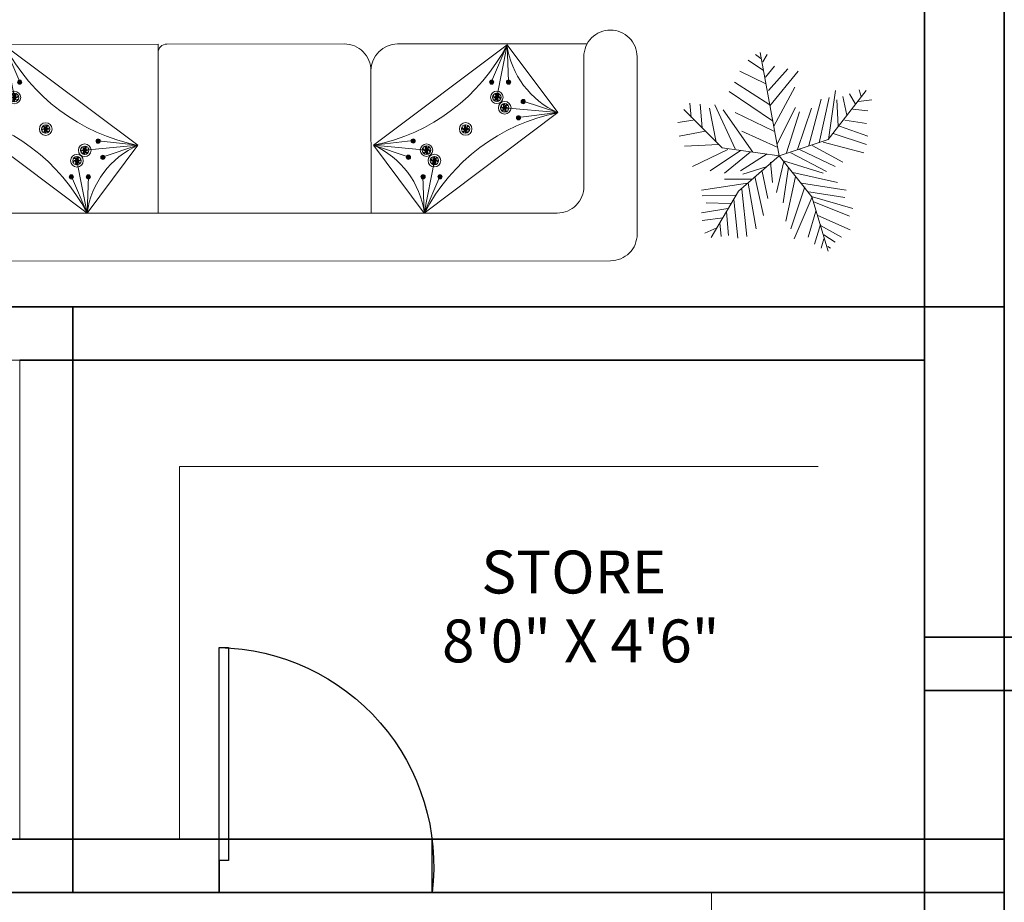
# Model space of a CAD drawing. Units: inches. Extents: x -61 to 1599, y -1316 to 257.
# Tile 23 of 204: x 434 to 545, y -1011 to -912. Entities that reach past the tile are written whole.
import ezdxf

# ---------------------------------------------------------------- set-up
doc = ezdxf.new("R2010")
doc.units = ezdxf.units.IN
doc.header["$MEASUREMENT"] = 0
doc.linetypes.add('ACAD_ISO02W100', pattern=[15, 12, -3])
for name, color, linetype, lineweight in [('A-ANNO-DIMS', 2, 'Continuous', 18), ('A-AREA-IDEN', 1, 'Continuous', 18), ('A-FLOR-CASE', 8, 'Continuous', 18), ('A-WALL-JAMB', 4, 'ACAD_ISO02W100', 25), ('DOORS', 2, 'Continuous', 25), ('FURNITURE', 83, 'Continuous', 18), ('WALLS', 4, 'Continuous', 35)]:
    doc.layers.add(name, color=color, linetype=linetype, lineweight=lineweight)
doc.layers.add('FUR', color=83, linetype='Continuous')
doc.styles.get("Standard").update_dxf_attribs({"font": 'arial.ttf'})
doc.dimstyles.get("Standard").update_dxf_attribs({"dimtxt": 0.18, "dimasz": 0.18, "dimexe": 0.18, "dimexo": 0.0625, "dimgap": 0.09, "dimtad": 0, "dimtih": 1, "dimtoh": 1, "dimdec": 0, "dimzin": 0, "dimdsep": 46, "dimlunit": 3, "dimtxsty": 'Standard', "dimcen": 0.09, "dimadec": 0, "dimazin": 0, "dimtfac": 1, "dimtdec": 0, "dimtofl": 0, "dimtmove": 0, "dimatfit": 3, "dimfxl": 1, "dimtolj": 1, "dimtzin": 0, "dimarcsym": 0})

# ---------------------------------------------------------------- blocks, each defined once
blk = doc.blocks.new('*U264')
for p, q in [((-10.186, 53.64), (-13.084, 55.962)), ((0, 0), (-10.5, 57)), ((-9.099, 51.782), (-6.563, 55.962)), ((-8.737, 47.138), (-17.069, 52.711)), ((-7.65, 43.423), (-2.578, 49.46)), ((-7.288, 39.707), (-21.778, 46.673)), ((-5.839, 35.992), (4.667, 48.067)), ((-5.114, 27.632), (10.463, 46.673)), ((-5.114, 28.097), (-24.676, 40.636)), ((-3.665, 19.273), (-27.574, 35.527)), ((-2.941, 16.486), (8.652, 37.85)), ((27, 9), (48, 36)), ((27.127, 9.056), (31.112, 35.992)), ((35.096, 32.741), (37.27, 22.524)), ((38.719, 34.134), (41.979, 28.561)), ((44.153, 36.456), (45.239, 32.741)), ((-48.585, 21.131), (-49.309, 29.026)), ((-43.513, 28.561), (-42.427, 15.558)), ((-35.544, 28.097), (-24.314, 3.947)), ((16.259, 5.805), (23.142, 31.348)), ((22.055, 7.198), (27.489, 32.277)), ((31.836, 30.883), (32.561, 16.486)), ((43.791, 29.954), (51.036, 30.883)), ((-31.5, 4.5), (-52.5, 25.5)), ((-38.442, 26.239), (-34.819, 7.663)), ((-14.533, 2.09), (-30.834, 25.31)), ((-24.314, 23.917), (-2.941, 13.7)), ((-1.129, 6.734), (9.014, 26.704)), ((3.942, 1.625), (11.187, 24.381)), ((10.101, 3.483), (17.708, 26.239)), ((40.53, 25.775), (48.862, 24.846)), ((-47.498, 19.737), (-55.83, 18.344)), ((33.285, 16.486), (48.862, 10.913)), ((36.183, 19.737), (48.137, 17.88)), ((-40.615, 13.7), (-55.105, 10.913)), ((-20.691, 13.7), (-1.129, 4.876)), ((29.662, 12.307), (48.137, 6.269)), ((-33.37, 6.269), (-52.207, 5.34)), ((0, 0), (27, 9)), ((18.07, 5.805), (35.096, -3.483)), ((24.229, 7.663), (46.688, 1.625)), ((-28.299, 3.483), (-47.86, -5.805)), ((-21.416, 3.018), (-38.079, -8.128)), ((0, 0), (-31.5, 4.5)), ((-15.982, 2.09), (-30.11, -9.521)), ((0, 0), (-22.5, -19.5)), ((-6.563, 1.161), (-21.416, -8.128)), ((0, 0), (18, -22.5)), ((6.478, 1.625), (26.04, -8.592)), ((11.187, 3.483), (30.749, -5.805)), ((-4.752, -3.483), (-3.665, -14.629)), ((2.493, -3.019), (-1.491, -20.202)), ((1.769, -2.555), (24.229, -9.521)), ((-6.563, -5.805), (-19.967, -9.985)), ((-9.461, -8.592), (-6.201, -23.453)), ((5.029, -6.27), (2.131, -25.775)), ((7.565, -9.056), (32.198, -14.629)), ((-17.431, -15.094), (-42.789, -18.809)), ((-15.257, -12.772), (-30.11, -12.772)), ((-17.069, -15.094), (-12.721, -40.172)), ((-13.446, -11.378), (-8.737, -32.741)), ((9.014, -11.378), (3.58, -35.992)), ((12.274, -15.094), (36.907, -18.809)), ((-24.314, -21.596), (-42.427, -22.06)), ((-22.5, -19.5), (-37.5, -45)), ((-20.691, -18.345), (-17.793, -44.352)), ((14.085, -16.951), (6.478, -40.172)), ((16.259, -19.738), (36.183, -22.989)), ((-26.849, -26.24), (-40.253, -25.775)), ((-25.038, -23.918), (-22.865, -45.281)), ((18.07, -22.524), (8.289, -45.745)), ((18, -22.5), (27, -52.5)), ((18.433, -22.524), (40.53, -29.026)), ((19.157, -25.311), (38.719, -33.206)), ((-28.299, -29.026), (-42.789, -31.348)), ((-29.023, -30.884), (-27.936, -43.887)), ((20.244, -30.419), (15.897, -44.816)), ((-30.834, -34.135), (-42.427, -35.528)), ((-32.646, -36.921), (-31.921, -44.352)), ((22.78, -37.85), (19.519, -48.532)), ((21.331, -32.741), (39.081, -40.636)), ((-34.457, -39.708), (-40.978, -42.494)), ((22.78, -38.314), (34.372, -44.816)), ((24.591, -45.745), (23.142, -50.854)), ((24.591, -43.423), (30.749, -47.603)), ((26.764, -49.925), (28.213, -50.854))]:
    blk.add_line(p, q)
blk = doc.blocks.new('DOOR-SWING-24')
blk.add_line((0, 0), (0, 3.6))
blk.add_lwpolyline([(0, 0), (0, -24), (1.05, -24), (1.05, 0)], close=True)
blk.add_arc((-0.44, 0.62), 24.62, 271.0259, 6.9559)
blk = doc.blocks.new('*U514')
at = {"layer": 'FUR'}
blk.add_open_spline([(0, 0.08), (-0.03, 0.05), (-0.1, -0.02), (0.08, -0.02), (0.02, -0.06), (0, -0.08)], degree=3, knots=[0, 0, 0, 0, 0.0954578, 0.1898773, 0.2470677, 0.2470677, 0.2470677, 0.2470677], dxfattribs=at)
blk = doc.blocks.new('*U515')
at = {"layer": 'FUR', "transparency": 16777216}
for p, rotation in [((222.17, -79.98), 60), ((222.31, -79.97), 300), ((222.18, -80.06), 120), ((222.25, -80.09), 180), ((222.32, -80.05), 240)]:
    blk.add_blockref('*U514', p, dxfattribs=dict(at, rotation=rotation))
blk.add_blockref('*U514', (222.24, -79.93), dxfattribs=at)
blk = doc.blocks.new('*U516')
at = {"layer": 'FUR'}
blk.add_open_spline([(0, 0.08), (-0.03, 0.05), (-0.1, -0.02), (0.08, -0.02), (0.02, -0.06), (0, -0.08)], degree=3, knots=[0, 0, 0, 0, 0.0954578, 0.1898773, 0.2470677, 0.2470677, 0.2470677, 0.2470677], dxfattribs=at)
blk = doc.blocks.new('*U517')
at = {"layer": 'FUR', "transparency": 16777216}
for p, rotation in [((222.17, -79.98), 60), ((222.31, -79.97), 300), ((222.18, -80.06), 120), ((222.25, -80.09), 180), ((222.32, -80.05), 240)]:
    blk.add_blockref('*U516', p, dxfattribs=dict(at, rotation=rotation))
blk.add_blockref('*U516', (222.24, -79.93), dxfattribs=at)
blk = doc.blocks.new('*U510')
at = {"layer": 'FUR'}
blk.add_open_spline([(0, 0.08), (-0.03, 0.05), (-0.1, -0.02), (0.08, -0.02), (0.02, -0.06), (0, -0.08)], degree=3, knots=[0, 0, 0, 0, 0.0954578, 0.1898773, 0.2470677, 0.2470677, 0.2470677, 0.2470677], dxfattribs=at)
blk = doc.blocks.new('*U511')
at = {"layer": 'FUR', "transparency": 16777216}
for p, rotation in [((222.17, -79.98), 60), ((222.31, -79.97), 300), ((222.18, -80.06), 120), ((222.25, -80.09), 180), ((222.32, -80.05), 240)]:
    blk.add_blockref('*U510', p, dxfattribs=dict(at, rotation=rotation))
blk.add_blockref('*U510', (222.24, -79.93), dxfattribs=at)
blk = doc.blocks.new('*U479')
at = {"layer": 'FUR'}
blk.add_open_spline([(0.01, 0.24), (-0.09, 0.14), (-0.29, -0.05), (0.22, -0.05), (0.07, -0.19), (0.01, -0.24)], degree=3, knots=[0, 0, 0, 0, 0.2846533, 0.5662105, 0.736751, 0.736751, 0.736751, 0.736751], dxfattribs=at)
blk = doc.blocks.new('*U480')
at = {"layer": 'FUR', "transparency": 16777216}
for p, rotation in [((662.52, -238.49), 60), ((662.53, -238.73), 120), ((662.74, -238.83), 180), ((662.93, -238.46), 300), ((662.94, -238.7), 240)]:
    blk.add_blockref('*U479', p, dxfattribs=dict(at, rotation=rotation))
blk.add_blockref('*U479', (662.72, -238.36), dxfattribs=at)
blk = doc.blocks.new('*U512')
at = {"layer": 'FUR'}
blk.add_open_spline([(0, 0.08), (-0.03, 0.05), (-0.1, -0.02), (0.08, -0.02), (0.02, -0.06), (0, -0.08)], degree=3, knots=[0, 0, 0, 0, 0.0954578, 0.1898773, 0.2470677, 0.2470677, 0.2470677, 0.2470677], dxfattribs=at)
blk = doc.blocks.new('*U513')
at = {"layer": 'FUR', "transparency": 16777216}
for p, rotation in [((222.17, -79.98), 60), ((222.31, -79.97), 300), ((222.18, -80.06), 120), ((222.25, -80.09), 180), ((222.32, -80.05), 240)]:
    blk.add_blockref('*U512', p, dxfattribs=dict(at, rotation=rotation))
blk.add_blockref('*U512', (222.24, -79.93), dxfattribs=at)
blk = doc.blocks.new('*U483')
at = {"layer": 'FUR'}
blk.add_open_spline([(0.01, 0.24), (-0.09, 0.14), (-0.29, -0.05), (0.22, -0.05), (0.07, -0.19), (0.01, -0.24)], degree=3, knots=[0, 0, 0, 0, 0.2846533, 0.5662105, 0.736751, 0.736751, 0.736751, 0.736751], dxfattribs=at)
blk = doc.blocks.new('*U484')
at = {"layer": 'FUR', "transparency": 16777216}
for p, rotation in [((662.52, -238.49), 60), ((662.53, -238.73), 120), ((662.74, -238.83), 180), ((662.93, -238.46), 300), ((662.94, -238.7), 240)]:
    blk.add_blockref('*U483', p, dxfattribs=dict(at, rotation=rotation))
blk.add_blockref('*U483', (662.72, -238.36), dxfattribs=at)
blk = doc.blocks.new('*U498')
at = {"layer": 'FUR'}
blk.add_open_spline([(0, 0.08), (-0.03, 0.05), (-0.1, -0.02), (0.08, -0.02), (0.02, -0.06), (0, -0.08)], degree=3, knots=[0, 0, 0, 0, 0.0954578, 0.1898773, 0.2470677, 0.2470677, 0.2470677, 0.2470677], dxfattribs=at)
blk = doc.blocks.new('*U499')
at = {"layer": 'FUR', "transparency": 16777216}
for p, rotation in [((222.17, -79.98), 60), ((222.31, -79.97), 300), ((222.18, -80.06), 120), ((222.25, -80.09), 180), ((222.32, -80.05), 240)]:
    blk.add_blockref('*U498', p, dxfattribs=dict(at, rotation=rotation))
blk.add_blockref('*U498', (222.24, -79.93), dxfattribs=at)
blk = doc.blocks.new('*U485')
at = {"layer": 'FUR'}
blk.add_open_spline([(0.01, 0.24), (-0.09, 0.14), (-0.29, -0.05), (0.22, -0.05), (0.07, -0.19), (0.01, -0.24)], degree=3, knots=[0, 0, 0, 0, 0.2846533, 0.5662105, 0.736751, 0.736751, 0.736751, 0.736751], dxfattribs=at)
blk = doc.blocks.new('*U497')
at = {"layer": 'FUR', "transparency": 16777216}
for p, rotation in [((662.52, -238.49), 60), ((662.53, -238.73), 120), ((662.74, -238.83), 180), ((662.93, -238.46), 300), ((662.94, -238.7), 240)]:
    blk.add_blockref('*U485', p, dxfattribs=dict(at, rotation=rotation))
blk.add_blockref('*U485', (662.72, -238.36), dxfattribs=at)
blk = doc.blocks.new('*U481')
at = {"layer": 'FUR'}
blk.add_open_spline([(0.01, 0.24), (-0.09, 0.14), (-0.29, -0.05), (0.22, -0.05), (0.07, -0.19), (0.01, -0.24)], degree=3, knots=[0, 0, 0, 0, 0.2846533, 0.5662105, 0.736751, 0.736751, 0.736751, 0.736751], dxfattribs=at)
blk = doc.blocks.new('*U482')
at = {"layer": 'FUR', "transparency": 16777216}
for p, rotation in [((662.52, -238.49), 60), ((662.53, -238.73), 120), ((662.74, -238.83), 180), ((662.93, -238.46), 300), ((662.94, -238.7), 240)]:
    blk.add_blockref('*U481', p, dxfattribs=dict(at, rotation=rotation))
blk.add_blockref('*U481', (662.72, -238.36), dxfattribs=at)
blk = doc.blocks.new('*U477')
at = {"layer": 'FUR'}
blk.add_open_spline([(0, 0.08), (-0.03, 0.05), (-0.1, -0.02), (0.08, -0.02), (0.02, -0.06), (0, -0.08)], degree=3, knots=[0, 0, 0, 0, 0.0954578, 0.1898773, 0.2470677, 0.2470677, 0.2470677, 0.2470677], dxfattribs=at)
blk = doc.blocks.new('*U478')
at = {"layer": 'FUR', "transparency": 16777216}
for p, rotation in [((222.17, -79.98), 60), ((222.31, -79.97), 300), ((222.18, -80.06), 120), ((222.25, -80.09), 180), ((222.32, -80.05), 240)]:
    blk.add_blockref('*U477', p, dxfattribs=dict(at, rotation=rotation))
blk.add_blockref('*U477', (222.24, -79.93), dxfattribs=at)
blk = doc.blocks.new('*U508')
at = {"layer": 'FUR'}
blk.add_open_spline([(0, 0.08), (-0.03, 0.05), (-0.1, -0.02), (0.08, -0.02), (0.02, -0.06), (0, -0.08)], degree=3, knots=[0, 0, 0, 0, 0.0954578, 0.1898773, 0.2470677, 0.2470677, 0.2470677, 0.2470677], dxfattribs=at)
blk = doc.blocks.new('*U509')
at = {"layer": 'FUR', "transparency": 16777216}
for p, rotation in [((222.17, -79.98), 60), ((222.31, -79.97), 300), ((222.18, -80.06), 120), ((222.25, -80.09), 180), ((222.32, -80.05), 240)]:
    blk.add_blockref('*U508', p, dxfattribs=dict(at, rotation=rotation))
blk.add_blockref('*U508', (222.24, -79.93), dxfattribs=at)
blk = doc.blocks.new('*U506')
at = {"layer": 'FUR'}
blk.add_open_spline([(0, 0.08), (-0.03, 0.05), (-0.1, -0.02), (0.08, -0.02), (0.02, -0.06), (0, -0.08)], degree=3, knots=[0, 0, 0, 0, 0.0954578, 0.1898773, 0.2470677, 0.2470677, 0.2470677, 0.2470677], dxfattribs=at)
blk = doc.blocks.new('*U507')
at = {"layer": 'FUR', "transparency": 16777216}
for p, rotation in [((222.17, -79.98), 60), ((222.31, -79.97), 300), ((222.18, -80.06), 120), ((222.25, -80.09), 180), ((222.32, -80.05), 240)]:
    blk.add_blockref('*U506', p, dxfattribs=dict(at, rotation=rotation))
blk.add_blockref('*U506', (222.24, -79.93), dxfattribs=at)
blk = doc.blocks.new('*U476')
at = {"layer": 'FUR'}
blk.add_open_spline([(0, 0.08), (-0.03, 0.05), (-0.1, -0.02), (0.08, -0.02), (0.02, -0.06), (0, -0.08)], degree=3, knots=[0, 0, 0, 0, 0.0954578, 0.1898773, 0.2470677, 0.2470677, 0.2470677, 0.2470677], dxfattribs=at)
blk = doc.blocks.new('*U489')
at = {"layer": 'FUR', "transparency": 16777216}
for p, rotation in [((222.17, -79.98), 60), ((222.31, -79.97), 300), ((222.18, -80.06), 120), ((222.25, -80.09), 180), ((222.32, -80.05), 240)]:
    blk.add_blockref('*U476', p, dxfattribs=dict(at, rotation=rotation))
blk.add_blockref('*U476', (222.24, -79.93), dxfattribs=at)
blk = doc.blocks.new('*U490')
at = {"layer": 'FUR'}
blk.add_open_spline([(0, 0.08), (-0.03, 0.05), (-0.1, -0.02), (0.08, -0.02), (0.02, -0.06), (0, -0.08)], degree=3, knots=[0, 0, 0, 0, 0.0954578, 0.1898773, 0.2470677, 0.2470677, 0.2470677, 0.2470677], dxfattribs=at)
blk = doc.blocks.new('*U491')
at = {"layer": 'FUR', "transparency": 16777216}
for p, rotation in [((222.17, -79.98), 60), ((222.31, -79.97), 300), ((222.18, -80.06), 120), ((222.25, -80.09), 180), ((222.32, -80.05), 240)]:
    blk.add_blockref('*U490', p, dxfattribs=dict(at, rotation=rotation))
blk.add_blockref('*U490', (222.24, -79.93), dxfattribs=at)
blk = doc.blocks.new('*U474')
at = {"layer": 'FUR'}
blk.add_open_spline([(0, 0.08), (-0.03, 0.05), (-0.1, -0.02), (0.08, -0.02), (0.02, -0.06), (0, -0.08)], degree=3, knots=[0, 0, 0, 0, 0.0954578, 0.1898773, 0.2470677, 0.2470677, 0.2470677, 0.2470677], dxfattribs=at)
blk = doc.blocks.new('*U475')
at = {"layer": 'FUR', "transparency": 16777216}
for p, rotation in [((222.17, -79.98), 60), ((222.31, -79.97), 300), ((222.18, -80.06), 120), ((222.25, -80.09), 180), ((222.32, -80.05), 240)]:
    blk.add_blockref('*U474', p, dxfattribs=dict(at, rotation=rotation))
blk.add_blockref('*U474', (222.24, -79.93), dxfattribs=at)
blk = doc.blocks.new('*U504')
at = {"layer": 'FUR'}
blk.add_open_spline([(0.01, 0.24), (-0.09, 0.14), (-0.29, -0.05), (0.22, -0.05), (0.07, -0.19), (0.01, -0.24)], degree=3, knots=[0, 0, 0, 0, 0.2846533, 0.5662105, 0.736751, 0.736751, 0.736751, 0.736751], dxfattribs=at)
blk = doc.blocks.new('*U505')
at = {"layer": 'FUR', "transparency": 16777216}
for p, rotation in [((662.52, -238.49), 60), ((662.53, -238.73), 120), ((662.74, -238.83), 180), ((662.93, -238.46), 300), ((662.94, -238.7), 240)]:
    blk.add_blockref('*U504', p, dxfattribs=dict(at, rotation=rotation))
blk.add_blockref('*U504', (662.72, -238.36), dxfattribs=at)
blk = doc.blocks.new('*U520')
at = {"layer": 'FUR'}
blk.add_open_spline([(0.01, 0.24), (-0.09, 0.14), (-0.29, -0.05), (0.22, -0.05), (0.07, -0.19), (0.01, -0.24)], degree=3, knots=[0, 0, 0, 0, 0.2846533, 0.5662105, 0.736751, 0.736751, 0.736751, 0.736751], dxfattribs=at)
blk = doc.blocks.new('*U471')
at = {"layer": 'FUR', "transparency": 16777216}
for p, rotation in [((662.52, -238.49), 60), ((662.53, -238.73), 120), ((662.74, -238.83), 180), ((662.93, -238.46), 300), ((662.94, -238.7), 240)]:
    blk.add_blockref('*U520', p, dxfattribs=dict(at, rotation=rotation))
blk.add_blockref('*U520', (662.72, -238.36), dxfattribs=at)
blk = doc.blocks.new('*U472')
at = {"layer": 'FUR'}
blk.add_open_spline([(0, 0.08), (-0.03, 0.05), (-0.1, -0.02), (0.08, -0.02), (0.02, -0.06), (0, -0.08)], degree=3, knots=[0, 0, 0, 0, 0.0954578, 0.1898773, 0.2470677, 0.2470677, 0.2470677, 0.2470677], dxfattribs=at)
blk = doc.blocks.new('*U473')
at = {"layer": 'FUR', "transparency": 16777216}
for p, rotation in [((222.17, -79.98), 60), ((222.31, -79.97), 300), ((222.18, -80.06), 120), ((222.25, -80.09), 180), ((222.32, -80.05), 240)]:
    blk.add_blockref('*U472', p, dxfattribs=dict(at, rotation=rotation))
blk.add_blockref('*U472', (222.24, -79.93), dxfattribs=at)
blk = doc.blocks.new('*U518')
at = {"layer": 'FUR'}
blk.add_open_spline([(0.01, 0.24), (-0.09, 0.14), (-0.29, -0.05), (0.22, -0.05), (0.07, -0.19), (0.01, -0.24)], degree=3, knots=[0, 0, 0, 0, 0.2846533, 0.5662105, 0.736751, 0.736751, 0.736751, 0.736751], dxfattribs=at)
blk = doc.blocks.new('*U519')
at = {"layer": 'FUR', "transparency": 16777216}
for p, rotation in [((662.52, -238.49), 60), ((662.53, -238.73), 120), ((662.74, -238.83), 180), ((662.93, -238.46), 300), ((662.94, -238.7), 240)]:
    blk.add_blockref('*U518', p, dxfattribs=dict(at, rotation=rotation))
blk.add_blockref('*U518', (662.72, -238.36), dxfattribs=at)
blk = doc.blocks.new('*U494')
at = {"layer": 'FUR'}
blk.add_open_spline([(0, 0.08), (-0.03, 0.05), (-0.1, -0.02), (0.08, -0.02), (0.02, -0.06), (0, -0.08)], degree=3, knots=[0, 0, 0, 0, 0.0954578, 0.1898773, 0.2470677, 0.2470677, 0.2470677, 0.2470677], dxfattribs=at)
blk = doc.blocks.new('*U495')
at = {"layer": 'FUR', "transparency": 16777216}
for p, rotation in [((222.17, -79.98), 60), ((222.31, -79.97), 300), ((222.18, -80.06), 120), ((222.25, -80.09), 180), ((222.32, -80.05), 240)]:
    blk.add_blockref('*U494', p, dxfattribs=dict(at, rotation=rotation))
blk.add_blockref('*U494', (222.24, -79.93), dxfattribs=at)
blk = doc.blocks.new('*U502')
at = {"layer": 'FUR'}
blk.add_open_spline([(0.01, 0.24), (-0.09, 0.14), (-0.29, -0.05), (0.22, -0.05), (0.07, -0.19), (0.01, -0.24)], degree=3, knots=[0, 0, 0, 0, 0.2846533, 0.5662105, 0.736751, 0.736751, 0.736751, 0.736751], dxfattribs=at)
blk = doc.blocks.new('*U503')
at = {"layer": 'FUR', "transparency": 16777216}
for p, rotation in [((662.52, -238.49), 60), ((662.53, -238.73), 120), ((662.74, -238.83), 180), ((662.93, -238.46), 300), ((662.94, -238.7), 240)]:
    blk.add_blockref('*U502', p, dxfattribs=dict(at, rotation=rotation))
blk.add_blockref('*U502', (662.72, -238.36), dxfattribs=at)
blk = doc.blocks.new('*U486')
at = {"layer": 'FUR'}
blk.add_open_spline([(0.01, 0.24), (-0.09, 0.14), (-0.29, -0.05), (0.22, -0.05), (0.07, -0.19), (0.01, -0.24)], degree=3, knots=[0, 0, 0, 0, 0.2846533, 0.5662105, 0.736751, 0.736751, 0.736751, 0.736751], dxfattribs=at)
blk = doc.blocks.new('*U487')
at = {"layer": 'FUR', "transparency": 16777216}
for p, rotation in [((662.52, -238.49), 60), ((662.53, -238.73), 120), ((662.74, -238.83), 180), ((662.93, -238.46), 300), ((662.94, -238.7), 240)]:
    blk.add_blockref('*U486', p, dxfattribs=dict(at, rotation=rotation))
blk.add_blockref('*U486', (662.72, -238.36), dxfattribs=at)
blk = doc.blocks.new('*U492')
at = {"layer": 'FUR'}
blk.add_open_spline([(0, 0.08), (-0.03, 0.05), (-0.1, -0.02), (0.08, -0.02), (0.02, -0.06), (0, -0.08)], degree=3, knots=[0, 0, 0, 0, 0.0954578, 0.1898773, 0.2470677, 0.2470677, 0.2470677, 0.2470677], dxfattribs=at)
blk = doc.blocks.new('*U493')
at = {"layer": 'FUR', "transparency": 16777216}
for p, rotation in [((222.17, -79.98), 60), ((222.31, -79.97), 300), ((222.18, -80.06), 120), ((222.25, -80.09), 180), ((222.32, -80.05), 240)]:
    blk.add_blockref('*U492', p, dxfattribs=dict(at, rotation=rotation))
blk.add_blockref('*U492', (222.24, -79.93), dxfattribs=at)
blk = doc.blocks.new('*U500')
at = {"layer": 'FUR'}
blk.add_open_spline([(0, 0.08), (-0.03, 0.05), (-0.1, -0.02), (0.08, -0.02), (0.02, -0.06), (0, -0.08)], degree=3, knots=[0, 0, 0, 0, 0.0954578, 0.1898773, 0.2470677, 0.2470677, 0.2470677, 0.2470677], dxfattribs=at)
blk = doc.blocks.new('*U501')
at = {"layer": 'FUR', "transparency": 16777216}
for p, rotation in [((222.17, -79.98), 60), ((222.31, -79.97), 300), ((222.18, -80.06), 120), ((222.25, -80.09), 180), ((222.32, -80.05), 240)]:
    blk.add_blockref('*U500', p, dxfattribs=dict(at, rotation=rotation))
blk.add_blockref('*U500', (222.24, -79.93), dxfattribs=at)
blk = doc.blocks.new('*U496')
at = {"layer": 'FUR'}
blk.add_open_spline([(0, 0.08), (-0.03, 0.05), (-0.1, -0.02), (0.08, -0.02), (0.02, -0.06), (0, -0.08)], degree=3, knots=[0, 0, 0, 0, 0.0954578, 0.1898773, 0.2470677, 0.2470677, 0.2470677, 0.2470677], dxfattribs=at)
blk = doc.blocks.new('*U488')
at = {"layer": 'FUR', "transparency": 16777216}
for p, rotation in [((222.17, -79.98), 60), ((222.31, -79.97), 300), ((222.18, -80.06), 120), ((222.25, -80.09), 180), ((222.32, -80.05), 240)]:
    blk.add_blockref('*U496', p, dxfattribs=dict(at, rotation=rotation))
blk.add_blockref('*U496', (222.24, -79.93), dxfattribs=at)
blk = doc.blocks.new('SOFA-THREE-SEAT-ALT-2')
for p, q in [((30, 24.44), (7, 24.38)), ((30, 23.44), (30, 24.44)), ((51, 24.44), (31, 24.44)), ((78.37, 24.44), (57, 24.44)), ((6, 23), (6, 23.38)), ((12.66, 24.33), (12.51, 20.19)), ((12.66, 24.33), (13.81, 18.42)), ((12.66, 24.33), (14.41, 20.19)), ((30, 23.44), (30, 5.38)), ((69.34, 24.33), (67.59, 20.19)), ((69.34, 24.33), (68.19, 18.42)), ((69.34, 24.33), (69.49, 20.19)), ((54, 21.44), (54, 5.38)), ((54, 21.44), (54, 21.44)), ((12.49, 20.14), (12.49, 20.3)), ((12.49, 20.14), (12.49, 19.98)), ((14.39, 20.14), (14.39, 20.3)), ((14.39, 20.14), (14.39, 19.98)), ((67.6, 20.14), (67.6, 20.3)), ((67.6, 20.14), (67.6, 19.98)), ((69.51, 20.14), (69.51, 20.3)), ((69.51, 20.14), (69.51, 19.98)), ((13.81, 18.42), (13.81, 18.9)), ((68.19, 18.42), (68.19, 18.9)), ((6.93, 16.69), (10.86, 17.99)), ((10.84, 17.94), (10.84, 18.1)), ((10.84, 17.94), (10.84, 17.78)), ((13.81, 18.42), (13.81, 17.95)), ((68.19, 18.42), (68.19, 17.95)), ((75.07, 16.69), (71.14, 17.99)), ((71.16, 17.94), (71.16, 18.1)), ((71.16, 17.94), (71.16, 17.78)), ((6.93, 16.69), (12.92, 17.24)), ((6.93, 16.69), (11.39, 16.16)), ((69.08, 17.24), (69.08, 17.72)), ((75.07, 16.69), (69.08, 17.24)), ((69.08, 17.24), (69.08, 16.77)), ((75.07, 16.69), (70.61, 16.16)), ((11.37, 16.11), (11.37, 16.27)), ((11.37, 16.11), (11.37, 15.95)), ((70.63, 16.11), (70.63, 16.27)), ((70.63, 16.11), (70.63, 15.95)), ((17.33, 14.86), (17.33, 15.33)), ((17.33, 14.86), (17.33, 14.38)), ((64.67, 14.86), (64.67, 15.33)), ((64.67, 14.86), (64.67, 14.38)), ((23.24, 13.5), (23.24, 13.66)), ((23.24, 13.5), (23.24, 13.34)), ((27.73, 13.03), (23.26, 13.55)), ((54.27, 13.03), (58.74, 13.55)), ((58.76, 13.5), (58.76, 13.66)), ((58.76, 13.5), (58.76, 13.34)), ((27.73, 13.03), (21.73, 12.47)), ((21.73, 12.47), (21.73, 12.95)), ((21.73, 12.47), (21.73, 12)), ((27.73, 13.03), (23.79, 11.72)), ((54.27, 13.03), (60.26, 12.47)), ((54.27, 13.03), (58.2, 11.72)), ((60.26, 12.47), (60.26, 12.95)), ((60.26, 12.47), (60.26, 12)), ((20.85, 11.29), (20.85, 11.77)), ((21.99, 5.38), (20.85, 11.29)), ((20.85, 11.29), (20.85, 10.82)), ((23.78, 11.67), (23.78, 11.83)), ((23.78, 11.67), (23.78, 11.51)), ((58.22, 11.67), (58.22, 11.83)), ((58.22, 11.67), (58.22, 11.51)), ((60.01, 5.38), (61.15, 11.29)), ((61.15, 11.29), (61.15, 11.77)), ((61.15, 11.29), (61.15, 10.82)), ((20.22, 9.47), (20.22, 9.63)), ((20.22, 9.47), (20.22, 9.31)), ((21.99, 5.38), (20.24, 9.52)), ((21.99, 5.38), (22.14, 9.52)), ((22.13, 9.47), (22.13, 9.63)), ((22.13, 9.47), (22.13, 9.31)), ((60.01, 5.38), (59.85, 9.52)), ((59.87, 9.47), (59.87, 9.63)), ((59.87, 9.47), (59.87, 9.31)), ((60.01, 5.38), (61.76, 9.52)), ((61.78, 9.47), (61.78, 9.63)), ((61.78, 9.47), (61.78, 9.31))]:
    blk.add_line(p, q)
blk.add_lwpolyline([(78, 8.38), (78, 23, -0.414214), (81, 26), (81, 26, -0.414214), (84, 23), (84, 3, -0.414214), (81, 0), (3, 0, -0.414214), (0, 3), (0, 23, -0.414214), (3, 26), (3, 26, -0.414214), (6, 23), (6, 8.38, 0.414214), (9, 5.38), (75, 5.38, 0.414214)], format="xyb", close=True)
for points in [[(27.73, 13.03), (12.66, 24.33), (6.93, 16.69), (21.99, 5.38)], [(54.27, 13.03), (69.34, 24.33), (75.07, 16.69), (60.01, 5.38)]]:
    blk.add_lwpolyline(points, close=True)
for centre, radius in [((12.49, 20.14), 0.238), ((12.49, 20.14), 0.16), ((14.39, 20.14), 0.238), ((14.39, 20.14), 0.16), ((67.6, 20.14), 0.238), ((67.6, 20.14), 0.16), ((69.51, 20.14), 0.238), ((69.51, 20.14), 0.16), ((13.81, 18.42), 0.71), ((13.81, 18.42), 0.476), ((68.19, 18.42), 0.71), ((68.19, 18.42), 0.476), ((10.84, 17.94), 0.238), ((10.84, 17.94), 0.16), ((69.08, 17.24), 0.71), ((71.16, 17.94), 0.238), ((71.16, 17.94), 0.16), ((69.08, 17.24), 0.476), ((11.37, 16.11), 0.238), ((11.37, 16.11), 0.16), ((17.33, 14.86), 0.71), ((64.67, 14.86), 0.71), ((70.63, 16.11), 0.238), ((70.63, 16.11), 0.16), ((17.33, 14.86), 0.476), ((64.67, 14.86), 0.476), ((23.24, 13.5), 0.238), ((23.24, 13.5), 0.16), ((58.76, 13.5), 0.238), ((58.76, 13.5), 0.16), ((21.73, 12.47), 0.71), ((21.73, 12.47), 0.476), ((60.26, 12.47), 0.71), ((60.26, 12.47), 0.476), ((20.85, 11.29), 0.71), ((20.85, 11.29), 0.476), ((23.78, 11.67), 0.238), ((23.78, 11.67), 0.16), ((58.22, 11.67), 0.238), ((58.22, 11.67), 0.16), ((61.15, 11.29), 0.71), ((61.15, 11.29), 0.476), ((20.22, 9.47), 0.238), ((20.22, 9.47), 0.16), ((22.13, 9.47), 0.238), ((22.13, 9.47), 0.16), ((59.87, 9.47), 0.238), ((59.87, 9.47), 0.16), ((61.78, 9.47), 0.238), ((61.78, 9.47), 0.16)]:
    blk.add_circle(centre, radius)
for centre, radius, start, end in [((31, 23.44), 1, 90, 180), ((51, 21.44), 3, 360, 90), ((57, 21.44), 3, 90, 180), ((7, 23.38), 1, 90.1542, 180.1542), ((2.94, 25.66), 9.82, 293.9742, 352.253), ((31.95, 34.34), 21.73, 207.4316, 258.7956), ((50.05, 34.34), 21.73, 281.2044, 332.5684), ((79.06, 25.66), 9.82, 187.747, 246.0258), ((2.7, -4.63), 21.73, 27.4316, 78.7956), ((79.3, -4.63), 21.73, 101.2044, 152.5684), ((31.72, 4.06), 9.82, 113.9742, 172.253), ((50.28, 4.06), 9.82, 7.747, 66.0258)]:
    blk.add_arc(centre, radius, start, end)
at = {"xscale": -1, "rotation": 180}
for name, p in [('*U511', (-209.75, -59.87)), ('*U513', (-207.85, -59.87)), ('*U480', (-648.93, -220.17)), ('*U515', (-211.41, -62.07)), ('*U517', (-210.87, -63.9)), ('*U484', (-645.4, -223.74)), ('*U509', (-199, -66.51)), ('*U482', (-641, -226.12)), ('*U497', (-641.88, -227.3)), ('*U507', (-198.47, -68.34)), ('*U499', (-202.02, -70.54)), ('*U478', (-200.12, -70.54))]:
    blk.add_blockref(name, p, dxfattribs=at)
at = {"rotation": 180}
for name, p in [('*U495', (289.85, -59.87)), ('*U493', (291.75, -59.87)), ('*U503', (730.92, -220.17)), ('*U488', (293.4, -62.07)), ('*U487', (731.81, -221.35)), ('*U501', (292.87, -63.9)), ('*U519', (727.4, -223.74)), ('*U491', (281, -66.51)), ('*U505', (722.99, -226.12)), ('*U489', (280.47, -68.34)), ('*U471', (723.88, -227.3)), ('*U475', (282.12, -70.54)), ('*U473', (284.02, -70.54))]:
    blk.add_blockref(name, p, dxfattribs=at)
blk = doc.blocks.new('*D696')
at = {"layer": 'A-ANNO-DIMS', "color": 0, "lineweight": -2, "transparency": 16777216}
for p, q in [((690.64, -873.17), (-61.08, -873.17)), ((-60.9, -873.35), (-60.9, -1025.8)), ((-60.9, -1178.61), (-60.9, -1026.16)), ((690.64, -1178.79), (-61.08, -1178.79))]:
    blk.add_line(p, q, dxfattribs=at)
at = {"layer": 'A-ANNO-DIMS', "color": 0, "transparency": 16777216}
for points in [[(-60.93, -873.35), (-60.87, -873.35), (-60.9, -873.17)], [(-60.93, -1178.61), (-60.87, -1178.61), (-60.9, -1178.79)]]:
    blk.add_solid(points, dxfattribs=at)
at = {"layer": 'DEFPOINTS', "color": 0, "transparency": 16777216}
for p in [(-60.9, -873.17), (690.7, -873.17), (690.7, -1178.79)]:
    blk.add_point(p, dxfattribs=at)
at = {"layer": 'A-ANNO-DIMS', "color": 0, "transparency": 16777216, "insert": (-60.9, -1025.98), "char_height": 0.18, "attachment_point": 5}
blk.add_mtext('\\A1;305.6', dxfattribs=at)

msp = doc.modelspace()

# ---------------------------------------------------------------- linework, layer by layer
at = {"layer": 'A-FLOR-CASE'}
for p, q in [((451.7028, -961.9446), (523.7028, -961.9446)), ((451.7028, -991.9446), (451.7028, -961.9446)), ((451.7028, -1003.9446), (451.7028, -991.9446)), ((511.7028, -1009.9446), (511.7028, -1033.9446))]:
    msp.add_line(p, q, dxfattribs=at)
msp.add_lwpolyline([(433.7028, -1003.9446), (421.7505, -1003.9446), (421.7505, -949.9446), (433.7028, -949.9446)], close=True, dxfattribs=at)
at = {"layer": 'A-WALL-JAMB'}
for p, q in [((456.2028, -1009.9446), (456.2028, -1003.9446)), ((480.2028, -1009.9446), (480.1983, -1003.9446))]:
    msp.add_line(p, q, dxfattribs=at)
at = {"layer": 'WALLS'}
for p, q in [((535.7028, -1215.9446), (535.7028, -741.169)), ((544.7028, -1215.9446), (544.7028, -741.169)), ((397.7028, -943.9446), (544.7028, -943.9446)), ((439.7028, -1009.9446), (439.7028, -943.9446)), ((433.7028, -949.9446), (439.7028, -949.9446)), ((439.7028, -949.9446), (535.7028, -949.9446)), ((535.7028, -981.169), (690.7028, -981.169)), ((535.7028, -987.169), (690.7028, -987.169)), ((367.7028, -1003.9446), (544.7028, -1003.9446)), ((433.7028, -1003.9446), (544.7028, -1003.9446)), ((367.7028, -1009.9446), (544.7028, -1009.9446)), ((433.7028, -1009.9446), (544.7028, -1009.9446))]:
    msp.add_line(p, q, dxfattribs=at)

# ---------------------------------------------------------------- block references
at = {"layer": 'DOORS', "extrusion": (0, 0, -1), "zscale": -1, "rotation": 180}
msp.add_blockref('DOOR-SWING-24', (-456.2028, -1006.3446), dxfattribs=at)
at = {"layer": 'FURNITURE', "rotation": 0.0183708733775309}
msp.add_blockref('SOFA-THREE-SEAT-ALT-2', (419.3112, -938.7885), dxfattribs=at)
at = {"layer": 'FURNITURE', "xscale": 0.2045054661246738, "yscale": 0.2045054661246738, "zscale": 0.2045054661246738}
msp.add_blockref('*U264', (519.3277, -926.9484), dxfattribs=at)

# ---------------------------------------------------------------- texts
at = {"layer": 'A-AREA-IDEN'}
for s, height, p in [('   STORE', 4.8321, (481.3179, -976.248)), ('8\'0" X 4\'6"', 4.832098, (481.3179, -984.0103))]:
    msp.add_text(s, height=height, dxfattribs=at).set_placement(p)

# ---------------------------------------------------------------- dimensions: what is measured, and where the dimension line sits
at = {"layer": 'A-ANNO-DIMS'}
dim = msp.add_linear_dim(base=(-60.8972, -873.169), p1=(690.7028, -1178.7933), p2=(690.7028, -873.169), angle=90, dimstyle='Standard', override={"dimdec": 1, "dimlfac": 1, "dimrnd": 0, "dimzin": 0, "dimdsep": 46, "dimlunit": 2}, dxfattribs=at)
dim.commit()
dim.dimension.update_dxf_attribs({"geometry": '*D696', "text_midpoint": (-60.8972, -1025.9812)})

doc.saveas('drawing.dxf')
